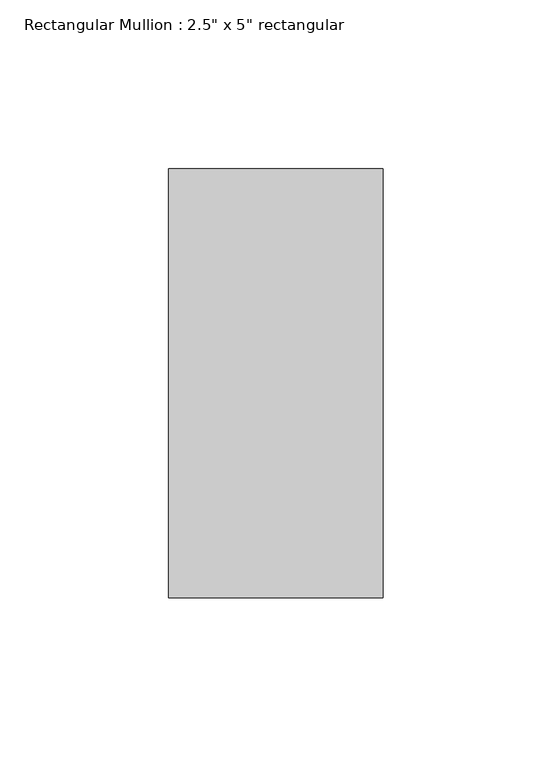
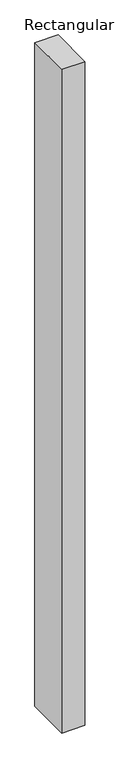
"""IFC4 building model written with IfcOpenShell, lengths in millimetres: member geometry."""

from ifc_helpers import new_model, si_unit, frame, origin, place, context, project, spatial, polyline, outline, extrude, source, transform, mapped, element, save


def member_995c57f6(model_context):
    return source(origin(), model_context, "Body", "SweptSolid", [
        extrude(outline(polyline([(0.0, 63.5), (0.0, -63.5), (-63.5, -63.5), (-63.5, 63.5), (0.0, 63.5)])), frame((0.0, 0.0, -1917.7), z_axis=(0.0, 0.0, 1.0), x_axis=(1.0, 0.0, 0.0)), (0.0, 0.0, 1.0), 1917.7),
    ])


if __name__ == "__main__":
    model = new_model("IFC4")
    model_context = context("Model", 3, world=origin())
    ifc_project = project(units=[si_unit("LENGTHUNIT", "METRE", prefix="MILLI")], contexts=[model_context])
    site = spatial("IfcSite", under=ifc_project)
    building = spatial("IfcBuilding", under=site)
    placement = place(None, origin())
    member_shape = member_995c57f6(model_context)
    element("IfcMember", 1, ObjectType="Rectangular Mullion : 2.5\" x 5\" rectangular", at=placement, inside=building, context=model_context, shape_type="MappedRepresentation", body=[
        mapped(member_shape, transform((0.0, 0.0, 0.0), x_axis=(1.0, 0.0, 0.0), y_axis=(0.0, 1.0, 0.0), z_axis=(0.0, 0.0, 1.0))),
    ])
    save(model, "model.ifc")

# Revit data of these elements
# Type "Rectangular Mullion : 2.5\" x 5\" rectangular"
#   built-in parameter 1007304 = 0.416667 (stored number, unit not read)
#   built-in parameter 1007301 = 0.104167 (stored number, unit not read)
#   built-in parameter 1007300 = 0.104167 (stored number, unit not read)
# Element 1 (IfcMember, "Rectangular Mullion : 2.5\" x 5\" rectangular")
#   Materials on its faces: "Aluminum"
# Materials
#   "Aluminum": class "Metal", colour RGB 247 247 247, transparency 0, Description = "Aluminum 6061", Cost = 0
